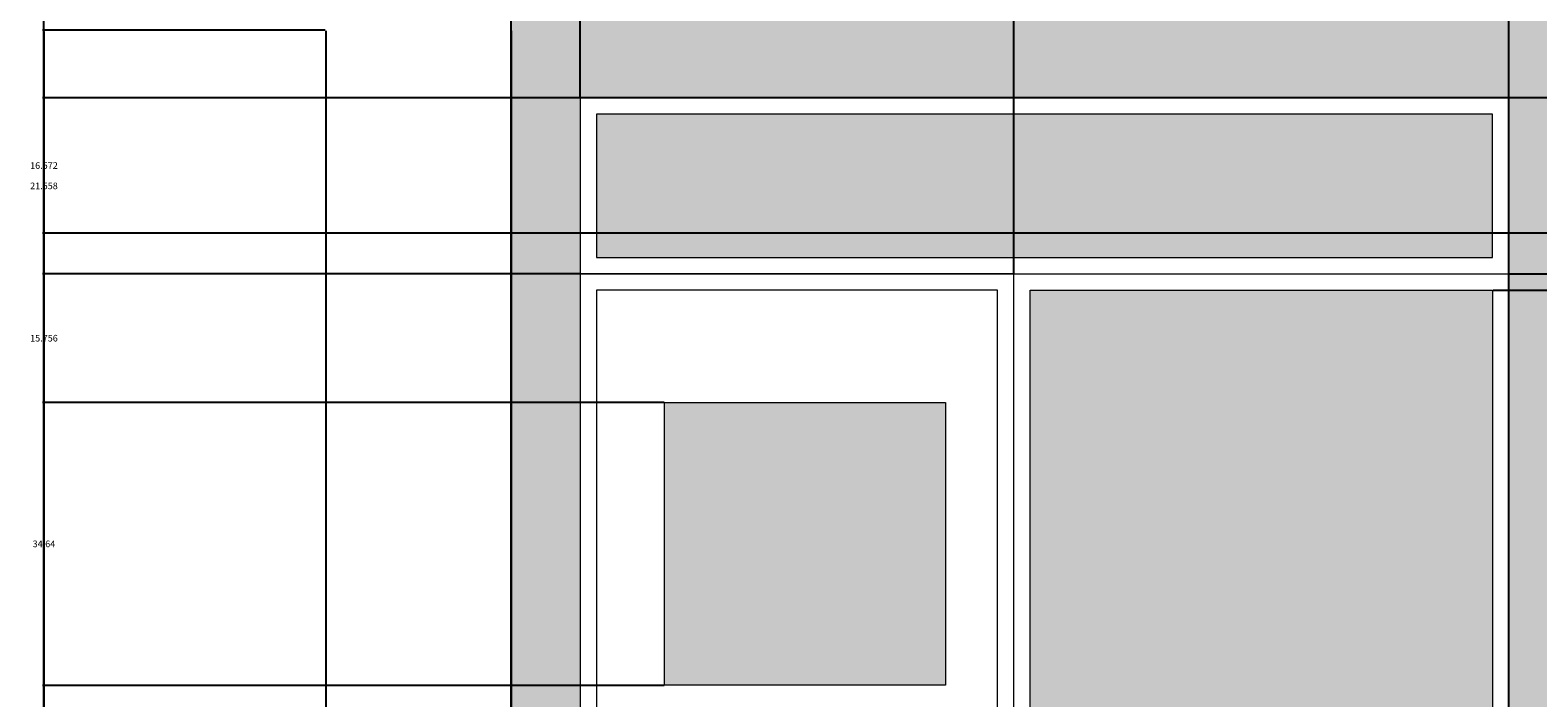
# Model space of a CAD drawing. Units: inches. Extents: x 36 to 594, y 79 to 831.
# Tile 3 of 30: x 36 to 221, y 213 to 294. Entities that reach past the tile are written whole.
import ezdxf

# ---------------------------------------------------------------- set-up
doc = ezdxf.new("R2010")
doc.units = ezdxf.units.IN
doc.header["$MEASUREMENT"] = 0
for name, color, linetype, lineweight in [('A-ANNO-DIMS', 2, 'Continuous', 18), ('A-DOOR', 3, 'Continuous', 18), ('A-ELEV', 7, 'Continuous', 25), ('A-ELEV-PATT', 8, 'Continuous', 13)]:
    doc.layers.add(name, color=color, linetype=linetype, lineweight=lineweight)
doc.styles.get("Standard").update_dxf_attribs({"font": 'arial.ttf'})
doc.dimstyles.get("Standard").update_dxf_attribs({"dimtxt": 0.8125, "dimasz": 0.18, "dimexe": 0.18, "dimexo": 0.0625, "dimgap": 0.09, "dimtad": 0, "dimtih": 1, "dimtoh": 1, "dimdec": 4, "dimzin": 0, "dimdsep": 46, "dimlunit": 4, "dimtxsty": 'Standard', "dimcen": 0.09, "dimadec": 0, "dimazin": 0, "dimtfac": 1, "dimtdec": 4, "dimtofl": 0, "dimtmove": 0, "dimatfit": 3, "dimfxl": 1, "dimtolj": 1, "dimtzin": 0, "dimarcsym": 0})

# ---------------------------------------------------------------- blocks, each defined once
blk = doc.blocks.new('*D28')
at = {"layer": 'A-ANNO-DIMS', "color": 0, "lineweight": -2, "transparency": 16777216}
for p, q in [((269.3, 796.05), (37.49, 796.05)), ((37.67, 795.87), (37.67, 455.63)), ((37.67, 114.39), (37.67, 454.62)), ((94.8, 114.21), (37.49, 114.21))]:
    blk.add_line(p, q, dxfattribs=at)
at = {"layer": 'A-ANNO-DIMS', "color": 0, "transparency": 16777216}
for points in [[(37.64, 795.87), (37.7, 795.87), (37.67, 796.05)], [(37.64, 114.39), (37.7, 114.39), (37.67, 114.21)]]:
    blk.add_solid(points, dxfattribs=at)
at = {"layer": 'Defpoints', "color": 0, "transparency": 16777216}
for p in [(37.67, 796.05), (269.36, 796.05), (94.87, 114.21)]:
    blk.add_point(p, dxfattribs=at)
at = {"layer": 'A-ANNO-DIMS', "color": 0, "transparency": 16777216, "insert": (37.67, 455.13), "char_height": 0.812, "attachment_point": 5}
blk.add_mtext('\\A1;681.8', dxfattribs=at)
blk = doc.blocks.new('*D42')
at = {"layer": 'A-ANNO-DIMS', "color": 0, "lineweight": -2, "transparency": 16777216}
for p, q in [((72.11, 294.48), (37.49, 294.48)), ((37.67, 294.3), (37.67, 204.85)), ((37.67, 114.39), (37.67, 203.84)), ((94.8, 114.21), (37.49, 114.21))]:
    blk.add_line(p, q, dxfattribs=at)
at = {"layer": 'A-ANNO-DIMS', "color": 0, "transparency": 16777216}
for points in [[(37.64, 294.3), (37.7, 294.3), (37.67, 294.48)], [(37.64, 114.39), (37.7, 114.39), (37.67, 114.21)]]:
    blk.add_solid(points, dxfattribs=at)
at = {"layer": 'Defpoints', "color": 0, "transparency": 16777216}
for p in [(37.67, 294.48), (72.17, 294.48), (94.87, 114.21)]:
    blk.add_point(p, dxfattribs=at)
at = {"layer": 'A-ANNO-DIMS', "color": 0, "transparency": 16777216, "insert": (37.67, 204.34), "char_height": 0.812, "attachment_point": 5}
blk.add_mtext('\\A1;180.26', dxfattribs=at)
blk = doc.blocks.new('*D43')
at = {"layer": 'A-ANNO-DIMS', "color": 0, "lineweight": -2, "transparency": 16777216}
for p, q in [((72.11, 422.59), (37.49, 422.59)), ((37.67, 422.41), (37.67, 359.04)), ((37.67, 294.66), (37.67, 358.03)), ((72.11, 294.48), (37.49, 294.48))]:
    blk.add_line(p, q, dxfattribs=at)
at = {"layer": 'A-ANNO-DIMS', "color": 0, "transparency": 16777216}
for points in [[(37.64, 422.41), (37.7, 422.41), (37.67, 422.59)], [(37.64, 294.66), (37.7, 294.66), (37.67, 294.48)]]:
    blk.add_solid(points, dxfattribs=at)
at = {"layer": 'Defpoints', "color": 0, "transparency": 16777216}
for p in [(37.67, 422.59), (72.17, 422.59), (72.17, 294.48)]:
    blk.add_point(p, dxfattribs=at)
at = {"layer": 'A-ANNO-DIMS', "color": 0, "transparency": 16777216, "insert": (37.67, 358.53), "char_height": 0.812, "attachment_point": 5}
blk.add_mtext('\\A1;128.1', dxfattribs=at)
blk = doc.blocks.new('*D53')
at = {"layer": 'A-ANNO-DIMS', "color": 0, "lineweight": -2, "transparency": 16777216}
for p, q in [((72.17, 294.41), (72.17, 79.53)), ((94.87, 294.41), (94.87, 79.53)), ((72.35, 79.71), (81.74, 79.71)), ((94.69, 79.71), (85.3, 79.71))]:
    blk.add_line(p, q, dxfattribs=at)
at = {"layer": 'A-ANNO-DIMS', "color": 0, "transparency": 16777216}
for points in [[(72.35, 79.74), (72.35, 79.68), (72.17, 79.71)], [(94.69, 79.74), (94.69, 79.68), (94.87, 79.71)]]:
    blk.add_solid(points, dxfattribs=at)
at = {"layer": 'Defpoints', "color": 0, "transparency": 16777216}
for p in [(72.17, 294.48), (94.87, 294.48), (94.87, 79.71)]:
    blk.add_point(p, dxfattribs=at)
at = {"layer": 'A-ANNO-DIMS', "color": 0, "transparency": 16777216, "insert": (83.52, 79.71), "char_height": 0.812, "attachment_point": 5}
blk.add_mtext('\\A1;22.692', dxfattribs=at)
blk = doc.blocks.new('*D60')
at = {"layer": 'A-ANNO-DIMS', "color": 0, "lineweight": -2, "transparency": 16777216}
for p, q in [((103.34, 286.24), (103.34, 830.73)), ((156.41, 264.68), (156.41, 830.73)), ((103.52, 830.55), (128.41, 830.55)), ((156.23, 830.55), (131.33, 830.55))]:
    blk.add_line(p, q, dxfattribs=at)
at = {"layer": 'A-ANNO-DIMS', "color": 0, "transparency": 16777216}
for points in [[(103.52, 830.58), (103.52, 830.52), (103.34, 830.55)], [(156.23, 830.58), (156.23, 830.52), (156.41, 830.55)]]:
    blk.add_solid(points, dxfattribs=at)
at = {"layer": 'Defpoints', "color": 0, "transparency": 16777216}
for p in [(156.41, 830.55), (103.34, 286.18), (156.41, 264.62)]:
    blk.add_point(p, dxfattribs=at)
at = {"layer": 'A-ANNO-DIMS', "color": 0, "transparency": 16777216, "insert": (129.87, 830.55), "char_height": 0.812, "attachment_point": 5}
blk.add_mtext('\\A1;53.07', dxfattribs=at)
blk = doc.blocks.new('*D61')
at = {"layer": 'A-ANNO-DIMS', "color": 0, "lineweight": -2, "transparency": 16777216}
for p, q in [((156.41, 264.68), (156.41, 830.73)), ((217.03, 286.24), (217.03, 830.73)), ((156.59, 830.55), (185.26, 830.55)), ((216.85, 830.55), (188.18, 830.55))]:
    blk.add_line(p, q, dxfattribs=at)
at = {"layer": 'A-ANNO-DIMS', "color": 0, "transparency": 16777216}
for points in [[(156.59, 830.58), (156.59, 830.52), (156.41, 830.55)], [(216.85, 830.58), (216.85, 830.52), (217.03, 830.55)]]:
    blk.add_solid(points, dxfattribs=at)
at = {"layer": 'Defpoints', "color": 0, "transparency": 16777216}
for p in [(217.03, 830.55), (217.03, 286.18), (156.41, 264.62)]:
    blk.add_point(p, dxfattribs=at)
at = {"layer": 'A-ANNO-DIMS', "color": 0, "transparency": 16777216, "insert": (186.72, 830.55), "char_height": 0.812, "attachment_point": 5}
blk.add_mtext('\\A1;60.62', dxfattribs=at)
blk = doc.blocks.new('*D70')
at = {"layer": 'A-ANNO-DIMS', "color": 0, "lineweight": -2, "transparency": 16777216}
for p, q in [((113.6, 214.22), (37.49, 214.22)), ((37.67, 214.04), (37.67, 209.15)), ((37.67, 203.24), (37.67, 208.14)), ((113.6, 203.06), (37.49, 203.06))]:
    blk.add_line(p, q, dxfattribs=at)
at = {"layer": 'A-ANNO-DIMS', "color": 0, "transparency": 16777216}
for points in [[(37.64, 214.04), (37.7, 214.04), (37.67, 214.22)], [(37.64, 203.24), (37.7, 203.24), (37.67, 203.06)]]:
    blk.add_solid(points, dxfattribs=at)
at = {"layer": 'Defpoints', "color": 0, "transparency": 16777216}
for p in [(37.67, 214.22), (113.66, 214.22), (113.66, 203.06)]:
    blk.add_point(p, dxfattribs=at)
at = {"layer": 'A-ANNO-DIMS', "color": 0, "transparency": 16777216, "insert": (37.67, 208.64), "char_height": 0.812, "attachment_point": 5}
blk.add_mtext('\\A1;11.167', dxfattribs=at)
blk = doc.blocks.new('*D71')
at = {"layer": 'A-ANNO-DIMS', "color": 0, "lineweight": -2, "transparency": 16777216}
for p, q in [((113.6, 248.87), (37.49, 248.87)), ((37.67, 248.69), (37.67, 232.05)), ((37.67, 214.4), (37.67, 231.04)), ((113.6, 214.22), (37.49, 214.22))]:
    blk.add_line(p, q, dxfattribs=at)
at = {"layer": 'A-ANNO-DIMS', "color": 0, "transparency": 16777216}
for points in [[(37.64, 248.69), (37.7, 248.69), (37.67, 248.87)], [(37.64, 214.4), (37.7, 214.4), (37.67, 214.22)]]:
    blk.add_solid(points, dxfattribs=at)
at = {"layer": 'Defpoints', "color": 0, "transparency": 16777216}
for p in [(37.67, 248.87), (113.66, 248.87), (113.66, 214.22)]:
    blk.add_point(p, dxfattribs=at)
at = {"layer": 'A-ANNO-DIMS', "color": 0, "transparency": 16777216, "insert": (37.67, 231.55), "char_height": 0.812, "attachment_point": 5}
blk.add_mtext('\\A1;34.64', dxfattribs=at)
blk = doc.blocks.new('*D72')
at = {"layer": 'A-ANNO-DIMS', "color": 0, "lineweight": -2, "transparency": 16777216}
for p, q in [((103.27, 264.62), (37.49, 264.62)), ((37.67, 264.44), (37.67, 257.25)), ((37.67, 249.05), (37.67, 256.24)), ((113.6, 248.87), (37.49, 248.87))]:
    blk.add_line(p, q, dxfattribs=at)
at = {"layer": 'A-ANNO-DIMS', "color": 0, "transparency": 16777216}
for points in [[(37.64, 264.44), (37.7, 264.44), (37.67, 264.62)], [(37.64, 249.05), (37.7, 249.05), (37.67, 248.87)]]:
    blk.add_solid(points, dxfattribs=at)
at = {"layer": 'Defpoints', "color": 0, "transparency": 16777216}
for p in [(37.67, 264.62), (103.34, 264.62), (113.66, 248.87)]:
    blk.add_point(p, dxfattribs=at)
at = {"layer": 'A-ANNO-DIMS', "color": 0, "transparency": 16777216, "insert": (37.67, 256.74), "char_height": 0.812, "attachment_point": 5}
blk.add_mtext('\\A1;15.756', dxfattribs=at)
blk = doc.blocks.new('*D73')
at = {"layer": 'A-ANNO-DIMS', "color": 0, "lineweight": -2, "transparency": 16777216}
for p, q in [((103.27, 286.18), (37.49, 286.18)), ((37.67, 286), (37.67, 275.91)), ((37.67, 264.8), (37.67, 274.9)), ((103.27, 264.62), (37.49, 264.62))]:
    blk.add_line(p, q, dxfattribs=at)
at = {"layer": 'A-ANNO-DIMS', "color": 0, "transparency": 16777216}
for points in [[(37.64, 286), (37.7, 286), (37.67, 286.18)], [(37.64, 264.8), (37.7, 264.8), (37.67, 264.62)]]:
    blk.add_solid(points, dxfattribs=at)
at = {"layer": 'Defpoints', "color": 0, "transparency": 16777216}
for p in [(37.67, 286.18), (103.34, 286.18), (103.34, 264.62)]:
    blk.add_point(p, dxfattribs=at)
at = {"layer": 'A-ANNO-DIMS', "color": 0, "transparency": 16777216, "insert": (37.67, 275.4), "char_height": 0.812, "attachment_point": 5}
blk.add_mtext('\\A1;21.558', dxfattribs=at)
blk = doc.blocks.new('*D75')
at = {"layer": 'A-ANNO-DIMS', "color": 0, "lineweight": -2, "transparency": 16777216}
for p, q in [((215.09, 262.62), (592.85, 262.62)), ((592.67, 262.44), (592.67, 221.53)), ((592.67, 179.6), (592.67, 220.52)), ((217.09, 179.42), (592.85, 179.42))]:
    blk.add_line(p, q, dxfattribs=at)
at = {"layer": 'A-ANNO-DIMS', "color": 0, "transparency": 16777216}
for points in [[(592.64, 262.44), (592.7, 262.44), (592.67, 262.62)], [(592.64, 179.6), (592.7, 179.6), (592.67, 179.42)]]:
    blk.add_solid(points, dxfattribs=at)
at = {"layer": 'Defpoints', "color": 0, "transparency": 16777216}
for p in [(215.03, 262.62), (592.67, 262.62), (217.03, 179.42)]:
    blk.add_point(p, dxfattribs=at)
at = {"layer": 'A-ANNO-DIMS', "color": 0, "transparency": 16777216, "insert": (592.67, 221.02), "char_height": 0.812, "attachment_point": 5}
blk.add_mtext('\\A1;83.2', dxfattribs=at)
blk = doc.blocks.new('*D76')
at = {"layer": 'A-ANNO-DIMS', "color": 0, "lineweight": -2, "transparency": 16777216}
for p, q in [((217.09, 264.62), (592.85, 264.62)), ((592.67, 264.44), (592.67, 264.12)), ((215.09, 262.62), (592.85, 262.62)), ((592.67, 262.8), (592.67, 263.12))]:
    blk.add_line(p, q, dxfattribs=at)
at = {"layer": 'A-ANNO-DIMS', "color": 0, "transparency": 16777216}
for points in [[(592.64, 264.44), (592.7, 264.44), (592.67, 264.62)], [(592.64, 262.8), (592.7, 262.8), (592.67, 262.62)]]:
    blk.add_solid(points, dxfattribs=at)
at = {"layer": 'Defpoints', "color": 0, "transparency": 16777216}
for p in [(217.03, 264.62), (592.67, 264.62), (215.03, 262.62)]:
    blk.add_point(p, dxfattribs=at)
at = {"layer": 'A-ANNO-DIMS', "color": 0, "transparency": 16777216, "insert": (592.67, 263.62), "char_height": 0.812, "attachment_point": 5}
blk.add_mtext('\\A1;2', dxfattribs=at)
blk = doc.blocks.new('*D90')
at = {"layer": 'A-ANNO-DIMS', "color": 0, "lineweight": -2, "transparency": 16777216}
for p, q in [((255.97, 269.61), (37.49, 269.61)), ((37.67, 269.43), (37.67, 210.78)), ((37.67, 151.11), (37.67, 209.77)), ((253.97, 150.93), (37.49, 150.93))]:
    blk.add_line(p, q, dxfattribs=at)
at = {"layer": 'A-ANNO-DIMS', "color": 0, "transparency": 16777216}
for points in [[(37.64, 269.43), (37.7, 269.43), (37.67, 269.61)], [(37.64, 151.11), (37.7, 151.11), (37.67, 150.93)]]:
    blk.add_solid(points, dxfattribs=at)
at = {"layer": 'Defpoints', "color": 0, "transparency": 16777216}
for p in [(37.67, 269.61), (256.03, 269.61), (254.03, 150.93)]:
    blk.add_point(p, dxfattribs=at)
at = {"layer": 'A-ANNO-DIMS', "color": 0, "transparency": 16777216, "insert": (37.67, 210.27), "char_height": 0.812, "attachment_point": 5}
blk.add_mtext('\\A1;118.67', dxfattribs=at)
blk = doc.blocks.new('*D91')
at = {"layer": 'A-ANNO-DIMS', "color": 0, "lineweight": -2, "transparency": 16777216}
for p, q in [((253.97, 286.18), (37.49, 286.18)), ((37.67, 286), (37.67, 278.4)), ((37.67, 269.79), (37.67, 277.39)), ((255.97, 269.61), (37.49, 269.61))]:
    blk.add_line(p, q, dxfattribs=at)
at = {"layer": 'A-ANNO-DIMS', "color": 0, "transparency": 16777216}
for points in [[(37.64, 286), (37.7, 286), (37.67, 286.18)], [(37.64, 269.79), (37.7, 269.79), (37.67, 269.61)]]:
    blk.add_solid(points, dxfattribs=at)
at = {"layer": 'Defpoints', "color": 0, "transparency": 16777216}
for p in [(37.67, 286.18), (254.03, 286.18), (256.03, 269.61)]:
    blk.add_point(p, dxfattribs=at)
at = {"layer": 'A-ANNO-DIMS', "color": 0, "transparency": 16777216, "insert": (37.67, 277.89), "char_height": 0.812, "attachment_point": 5}
blk.add_mtext('\\A1;16.572', dxfattribs=at)

msp = doc.modelspace()

# ---------------------------------------------------------------- hatches: boundary and pattern name
at = {"layer": 'A-ELEV-PATT'}
h = msp.add_hatch(color=256, dxfattribs=at)
h.dxf.hatch_style = 1
h.paths.add_polyline_path([(398.0873, 796.0465), (269.3592, 796.0465), (269.3592, 770.1455), (397.8159, 770.1455)])
h.paths.add_polyline_path([(397.7518, 764.0341), (269.3592, 764.0341), (269.3592, 630.0394), (341.8367, 630.0394), (341.8367, 720.595), (335.0881, 728.3699), (329.982, 735.3373), (345.3661, 727.7743), (397.1052, 702.3389)])
h.paths.add_polyline_path([(341.8367, 594.2124), (201.4189, 594.2124), (201.4189, 475.4136), (232.8216, 475.4136), (232.8216, 524.6037), (341.8367, 524.6037)])
h.paths.add_polyline_path([(177.525, 594.2124), (118.7598, 594.2124), (118.7598, 450.2124), (177.525, 450.2124)])
h.paths.add_polyline_path([(424.4958, 594.2124), (365.7306, 594.2124), (365.7306, 450.2124), (424.4958, 450.2124)])
h.paths.add_polyline_path([(241.3553, 404.2737), (355.8569, 404.2737), (355.8569, 355.0836), (424.5492, 355.0836), (424.5492, 425.7333), (118.7598, 426.2844), (118.7598, 355.0836), (241.3553, 355.0836)])
h.paths.add_polyline_path([(448.3898, 306.2124), (217.0273, 306.2124), (217.0273, 142.2124), (254.0293, 142.2124), (254.0293, 150.9347), (254.0293, 286.1802), (401.5491, 286.1802), (401.5491, 150.9347), (401.5491, 142.2124), (448.3898, 142.2124)])
h.paths.add_polyline_path([(448.3898, 142.2124), (401.5491, 142.2124), (217.0273, 142.2124), (217.0273, 114.2124), (448.3898, 114.2124)])
h.paths.add_polyline_path([(217.0273, 306.2124), (174.7353, 306.2124), (94.8658, 306.2124), (94.8658, 162.2124), (103.3368, 162.2124), (103.3368, 264.6224), (103.3368, 286.1802), (217.0273, 286.1802)])
h = msp.add_hatch(color=256, dxfattribs=at)
h.dxf.hatch_style = 1
h.set_gradient(color1=(0, 255, 255), color2=(16, 86, 137))
h.paths.add_polyline_path([(341.8367, 524.6037), (260.5056, 524.6037), (260.5056, 513.1224), (341.8367, 513.1224)])
h.paths.add_polyline_path([(341.8367, 511.1224), (260.5056, 511.1224), (260.5056, 475.4136), (341.8367, 475.4136)])
h.paths.add_polyline_path([(258.5056, 524.6037), (232.8216, 524.6037), (232.8216, 513.1224), (258.5056, 513.1224)])
h.paths.add_polyline_path([(355.8569, 404.2737), (269.0393, 404.2737), (269.0393, 392.7924), (355.8569, 392.7924)])
h.paths.add_polyline_path([(267.0393, 404.2737), (241.3553, 404.2737), (241.3553, 392.7924), (267.0393, 392.7924)])
h.paths.add_polyline_path([(355.8569, 390.7924), (269.0393, 390.7924), (269.0393, 355.0836), (355.8569, 355.0836)])
h.paths.add_polyline_path([(399.5491, 284.1802), (256.0293, 284.1802), (256.0293, 271.378), (399.5491, 271.378)])
h.paths.add_polyline_path([(317.3533, 259.1243), (262.3169, 259.1243), (262.3169, 200.6645), (317.3533, 200.6645)])
h.paths.add_polyline_path([(390.386, 259.1243), (335.3496, 259.1243), (335.3496, 200.6645), (390.386, 200.6645)])
h.paths.add_polyline_path([(390.386, 190.7697), (335.3496, 190.7697), (335.3496, 162.9881), (390.386, 162.9881)])
h.paths.add_polyline_path([(317.3533, 190.7697), (262.3169, 190.7697), (262.3169, 162.9881), (317.3533, 162.9881)])
h.paths.add_polyline_path([(215.0273, 262.6224), (158.4069, 262.6224), (158.4069, 181.4195), (215.0273, 181.4195)])
h.paths.add_polyline_path([(215.0273, 284.1802), (105.3368, 284.1802), (105.3368, 266.6224), (215.0273, 266.6224)])
h = msp.add_hatch(dxfattribs=at)
h.set_pattern_fill('ANSI33', color=256, scale=6.3, angle=135)
h.paths.add_polyline_path([(255.3555, 505.4499), (236.2911, 505.4499), (236.2911, 488.4928), (255.3555, 488.4928)])
h.paths.add_polyline_path([(255.3555, 484.4187), (236.2911, 484.4187), (236.2911, 475.4136), (255.3555, 475.4136)])
h.paths.add_polyline_path([(263.8892, 385.1199), (244.8248, 385.1199), (244.8248, 368.1628), (263.8892, 368.1628)])
h.paths.add_polyline_path([(263.8892, 364.0887), (244.8248, 364.0887), (244.8248, 355.0836), (263.8892, 355.0836)])
h.paths.add_polyline_path([(148.0383, 248.8663), (113.6593, 248.8663), (113.6593, 214.2237), (148.0383, 214.2237)])
h.paths.add_polyline_path([(148.0383, 203.057), (113.6593, 203.057), (113.6593, 170.5978), (148.0383, 170.5978)])

# ---------------------------------------------------------------- linework, layer by layer
at = {"layer": 'A-DOOR'}
for points in [[(103.3368, 264.6224), (217.0273, 264.6224), (217.0273, 286.1802), (103.3368, 286.1802)], [(105.3368, 266.6224), (215.0273, 266.6224), (215.0273, 284.1802), (105.3368, 284.1802)], [(103.3368, 162.2124), (156.4069, 162.2124), (156.4069, 264.6224), (103.3368, 264.6224)], [(156.4069, 264.6224), (217.0273, 264.6224), (217.0273, 179.4195), (156.4069, 179.4195)], [(105.3368, 164.2124), (154.4069, 164.2124), (154.4069, 262.6224), (105.3368, 262.6224)], [(158.4069, 262.6224), (215.0273, 262.6224), (215.0273, 181.4195), (158.4069, 181.4195)], [(113.6593, 248.8663), (148.0383, 248.8663), (148.0383, 214.2237), (113.6593, 214.2237)]]:
    msp.add_lwpolyline(points, close=True, dxfattribs=at)
at = {"layer": 'A-ELEV'}
for p, q in [((94.8658, 162.2124), (94.8658, 306.2124)), ((217.0273, 114.2124), (217.0273, 306.2124))]:
    msp.add_line(p, q, dxfattribs=at)

# ---------------------------------------------------------------- dimensions: what is measured, and where the dimension line sits
at = {"layer": 'A-ANNO-DIMS'}
for base, p1, p2, override, picture, middle in [((156.4069, 830.5465), (103.3368, 286.1802), (156.4069, 264.6224), {"dimdec": 2, "dimlfac": 1, "dimrnd": 0, "dimzin": 0, "dimdsep": 46, "dimlunit": 2}, '*D60', (129.8718, 830.5465)), ((217.0273, 830.5465), (156.4069, 264.6224), (217.0273, 286.1802), {"dimdec": 2, "dimlfac": 1, "dimrnd": 0, "dimzin": 0, "dimdsep": 46, "dimlunit": 2}, '*D61', (186.7171, 830.5465)), ((94.86583, 79.71236), (72.17334, 294.47595), (94.86583, 294.47595), {"dimdec": 3, "dimlfac": 1, "dimrnd": 0, "dimzin": 0, "dimdsep": 46, "dimlunit": 2}, '*D53', (83.51959, 79.71236))]:
    dim = msp.add_linear_dim(base=base, p1=p1, p2=p2, dimstyle='Standard', override=override, dxfattribs=at)
    dim.commit()
    dim.dimension.update_dxf_attribs({"geometry": picture, "text_midpoint": middle})
for base, p1, p2, override, picture, middle in [((37.6733, 796.0465), (94.8658, 114.2124), (269.3592, 796.0465), {"dimdec": 1, "dimlfac": 1, "dimrnd": 0, "dimzin": 0, "dimdsep": 46, "dimlunit": 2}, '*D28', (37.6733, 455.1294)), ((37.6733, 422.5882), (72.1733, 294.4759), (72.1733, 422.5882), {"dimdec": 1, "dimlfac": 1, "dimrnd": 0, "dimzin": 0, "dimdsep": 46, "dimlunit": 2}, '*D43', (37.6733, 358.5321)), ((37.6733, 294.4759), (94.8658, 114.2124), (72.1733, 294.4759), {"dimdec": 2, "dimlfac": 1, "dimrnd": 0, "dimzin": 0, "dimdsep": 46, "dimlunit": 2}, '*D42', (37.6733, 204.3442)), ((37.6733, 286.1802), (103.3368, 264.6224), (103.3368, 286.1802), {"dimdec": 3, "dimlfac": 1, "dimrnd": 0, "dimzin": 0, "dimdsep": 46, "dimlunit": 2}, '*D73', (37.6733, 275.4013)), ((37.6733, 286.1802), (256.0293, 269.6084), (254.0293, 286.1802), {"dimdec": 3, "dimlfac": 1, "dimrnd": 0, "dimzin": 0, "dimdsep": 46, "dimlunit": 2}, '*D91', (37.6733, 277.8943)), ((37.6733, 269.6084), (254.0293, 150.9347), (256.0293, 269.6084), {"dimdec": 2, "dimlfac": 1, "dimrnd": 0, "dimzin": 0, "dimdsep": 46, "dimlunit": 2}, '*D90', (37.6733, 210.2716)), ((37.6733, 264.6224), (113.6593, 248.8663), (103.3368, 264.6224), {"dimdec": 3, "dimlfac": 1, "dimrnd": 0, "dimzin": 0, "dimdsep": 46, "dimlunit": 2}, '*D72', (37.6733, 256.7444)), ((592.6689, 264.6224), (215.0273, 262.6224), (217.0273, 264.6224), {"dimdec": 0, "dimlfac": 1, "dimrnd": 0, "dimzin": 0, "dimdsep": 46, "dimlunit": 2}, '*D76', (592.6689, 263.6224)), ((592.6689, 262.6224), (217.0273, 179.4195), (215.0273, 262.6224), {"dimdec": 1, "dimlfac": 1, "dimrnd": 0, "dimzin": 0, "dimdsep": 46, "dimlunit": 2}, '*D75', (592.6689, 221.021)), ((37.6733, 248.8663), (113.6593, 214.2237), (113.6593, 248.8663), {"dimdec": 2, "dimlfac": 1, "dimrnd": 0, "dimzin": 0, "dimdsep": 46, "dimlunit": 2}, '*D71', (37.6733, 231.545)), ((37.6733, 214.2237), (113.6593, 203.057), (113.6593, 214.2237), {"dimdec": 3, "dimlfac": 1, "dimrnd": 0, "dimzin": 0, "dimdsep": 46, "dimlunit": 2}, '*D70', (37.6733, 208.6404))]:
    dim = msp.add_linear_dim(base=base, p1=p1, p2=p2, angle=90, dimstyle='Standard', override=override, dxfattribs=at)
    dim.commit()
    dim.dimension.update_dxf_attribs({"geometry": picture, "text_midpoint": middle})

doc.saveas('drawing.dxf')
